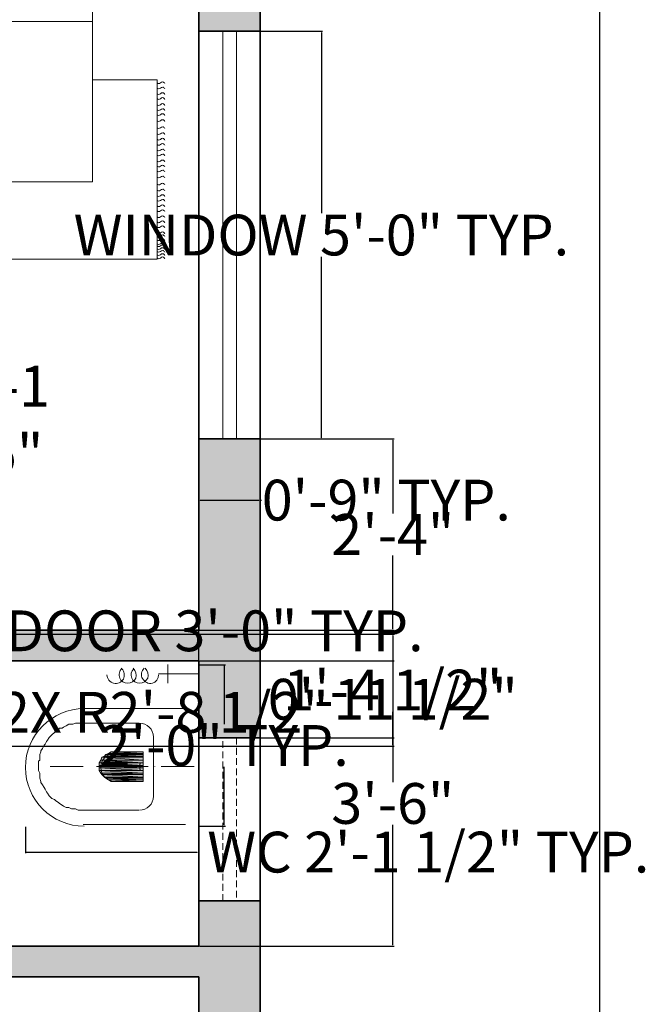
# Model space of a CAD drawing. Units: inches. Extents: x 335 to 688, y 1043 to 1486.
# Tile 6 of 7: x 596 to 688, y 1258 to 1403. Entities that reach past the tile are written whole.
import ezdxf

# ---------------------------------------------------------------- set-up
doc = ezdxf.new("R2010")
doc.units = ezdxf.units.IN
doc.header["$MEASUREMENT"] = 0
doc.linetypes.add('DASHEDX2', pattern=[1.5, 1, -0.5])
for name, color, linetype, lineweight in [('A-ANNO-DIMS', 2, 'Continuous', 18), ('A-ANNO-TTLB', 7, 'Continuous', 25), ('A-AREA-IDEN', 7, 'Continuous', 18), ('A-FLOR-FIXT', 8, 'Continuous', 18), ('A-FURN', 8, 'Continuous', 18), ('A-GLAZ', 4, 'Continuous', 18), ('A-GLAZ-VENT', 4, 'DASHEDX2', 18), ('A-WALL', 7, 'Continuous', 35), ('A-WALL-PATT', 252, 'Continuous', 13)]:
    doc.layers.add(name, color=color, linetype=linetype, lineweight=lineweight)
doc.styles.get("Standard").update_dxf_attribs({"font": 'arial.ttf'})
doc.dimstyles.get("Standard").update_dxf_attribs({"dimtxt": 6, "dimasz": 0.18, "dimexe": 0.18, "dimexo": 0.0625, "dimgap": 0.09, "dimtad": 0, "dimtih": 1, "dimtoh": 1, "dimdec": 1, "dimzin": 0, "dimdsep": 46, "dimlunit": 3, "dimtxsty": 'Standard', "dimcen": 0.09, "dimadec": 0, "dimazin": 0, "dimtfac": 1, "dimtdec": 1, "dimtofl": 0, "dimtmove": 0, "dimatfit": 3, "dimfxl": 1, "dimtolj": 1, "dimtzin": 0, "dimarcsym": 0})

# ---------------------------------------------------------------- blocks, each defined once
blk = doc.blocks.new('BED-DOUBLE-WITH-NIGHTSTANDS')
for p, q in [((56.59, 58.08), (56.59, 68.14)), ((0, 64.35), (26.37, 64.35)), ((0, 1.12), (0, 64.35)), ((26.37, 64.35), (26.37, 58.06)), ((61.62, 63.11), (51.56, 63.11)), ((34.96, 10.66), (34.96, 58.08)), ((52, 19.27), (52, 58.08)), ((52.82, 19.32), (52.82, 58.08)), ((52.82, 19.32), (46.47, 10.71)), ((52.82, 19.27), (46.47, 19.27)), ((46.47, 19.27), (46.47, 10.71)), ((26.37, 10.66), (26.37, 1.12)), ((56.69, 0.03), (56.69, 10.09)), ((61.72, 5.06), (51.66, 5.06)), ((26.37, 1.12), (0, 1.12))]:
    blk.add_line(p, q)
for points in [[(50.39, 68.71), (50.5, 58.08), (62.68, 58.08), (62.58, 68.71)], [(62.68, 10.66), (11.37, 10.66), (11.37, 58.08), (62.68, 58.08)], [(59.98, 38.83), (52.82, 38.83), (52.82, 52.73), (59.98, 52.73)], [(59.98, 19.27), (52.82, 19.27), (52.82, 33.16), (59.98, 33.16)], [(50.5, 10.66), (50.6, 0.03), (62.78, 0.03), (62.68, 10.66)]]:
    blk.add_lwpolyline(points, close=True)
for centre in [(56.59, 63.11), (56.69, 5.06)]:
    blk.add_circle(centre, 3.92)
for points, knots in [([(0.07, 65.48), (0.19, 65.39), (0.43, 65.19), (0.19, 64.85), (0.02, 64.57), (0.13, 64.42), (0.18, 64.35)], [0, 0, 0, 0, 0.400747, 0.791423, 1.067667, 1.29709, 1.29709, 1.29709, 1.29709]), ([(0.57, 65.48), (0.7, 65.39), (0.94, 65.19), (0.7, 64.85), (0.52, 64.57), (0.63, 64.42), (0.68, 64.35)], [0, 0, 0, 0, 0.400747, 0.791423, 1.067667, 1.29709, 1.29709, 1.29709, 1.29709]), ([(1.06, 65.48), (1.18, 65.39), (1.42, 65.19), (1.18, 64.85), (1.01, 64.57), (1.11, 64.42), (1.16, 64.35)], [0, 0, 0, 0, 0.400747, 0.791423, 1.067667, 1.29709, 1.29709, 1.29709, 1.29709]), ([(1.46, 65.48), (1.58, 65.39), (1.82, 65.19), (1.58, 64.85), (1.41, 64.57), (1.51, 64.42), (1.56, 64.35)], [0, 0, 0, 0, 0.400747, 0.791423, 1.067667, 1.29709, 1.29709, 1.29709, 1.29709]), ([(1.88, 65.48), (2, 65.39), (2.24, 65.19), (2, 64.85), (1.82, 64.57), (1.93, 64.42), (1.98, 64.35)], [0, 0, 0, 0, 0.400747, 0.791423, 1.067667, 1.29709, 1.29709, 1.29709, 1.29709]), ([(2.18, 65.48), (2.31, 65.39), (2.55, 65.19), (2.31, 64.85), (2.13, 64.57), (2.24, 64.42), (2.29, 64.35)], [0, 0, 0, 0, 0.400747, 0.791423, 1.067667, 1.29709, 1.29709, 1.29709, 1.29709]), ([(2.76, 65.48), (2.88, 65.39), (3.12, 65.19), (2.88, 64.85), (2.71, 64.57), (2.81, 64.42), (2.86, 64.35)], [0, 0, 0, 0, 0.400747, 0.791423, 1.067667, 1.29709, 1.29709, 1.29709, 1.29709]), ([(3.33, 65.48), (3.45, 65.39), (3.7, 65.19), (3.44, 64.85), (3.27, 64.57), (3.38, 64.42), (3.43, 64.35)], [0, 0, 0, 0, 0.407265, 0.802015, 1.07826, 1.307683, 1.307683, 1.307683, 1.307683]), ([(3.75, 65.48), (3.88, 65.39), (4.12, 65.19), (3.88, 64.85), (3.7, 64.57), (3.81, 64.42), (3.86, 64.35)], [0, 0, 0, 0, 0.400747, 0.791423, 1.067667, 1.29709, 1.29709, 1.29709, 1.29709]), ([(4.64, 65.48), (4.76, 65.39), (5, 65.19), (4.76, 64.85), (4.59, 64.57), (4.69, 64.42), (4.74, 64.35)], [0, 0, 0, 0, 0.400747, 0.791423, 1.067667, 1.29709, 1.29709, 1.29709, 1.29709]), ([(5.36, 65.48), (5.49, 65.39), (5.73, 65.19), (5.49, 64.85), (5.31, 64.57), (5.42, 64.42), (5.47, 64.35)], [0, 0, 0, 0, 0.400747, 0.791423, 1.067667, 1.29709, 1.29709, 1.29709, 1.29709]), ([(6.12, 65.48), (6.24, 65.39), (6.48, 65.19), (6.24, 64.85), (6.07, 64.57), (6.17, 64.42), (6.22, 64.35)], [0, 0, 0, 0, 0.400747, 0.791423, 1.067667, 1.29709, 1.29709, 1.29709, 1.29709]), ([(7, 65.48), (7.12, 65.39), (7.36, 65.19), (7.12, 64.85), (6.95, 64.57), (7.05, 64.42), (7.1, 64.35)], [0, 0, 0, 0, 0.400747, 0.791423, 1.067667, 1.29709, 1.29709, 1.29709, 1.29709]), ([(7.73, 65.48), (7.85, 65.39), (8.09, 65.19), (7.85, 64.85), (7.68, 64.57), (7.78, 64.42), (7.83, 64.35)], [0, 0, 0, 0, 0.400747, 0.791423, 1.067667, 1.29709, 1.29709, 1.29709, 1.29709]), ([(8.54, 65.48), (8.66, 65.39), (8.9, 65.19), (8.66, 64.85), (8.49, 64.57), (8.6, 64.42), (8.65, 64.35)], [0, 0, 0, 0, 0.400747, 0.791423, 1.067667, 1.29709, 1.29709, 1.29709, 1.29709]), ([(9.23, 65.48), (9.35, 65.39), (9.59, 65.19), (9.35, 64.85), (9.18, 64.57), (9.29, 64.42), (9.34, 64.35)], [0, 0, 0, 0, 0.400747, 0.791423, 1.067667, 1.29709, 1.29709, 1.29709, 1.29709]), ([(10.05, 65.48), (10.17, 65.39), (10.41, 65.19), (10.17, 64.85), (10, 64.57), (10.1, 64.42), (10.15, 64.35)], [0, 0, 0, 0, 0.400747, 0.791423, 1.067667, 1.29709, 1.29709, 1.29709, 1.29709]), ([(10.93, 65.48), (11.05, 65.39), (11.29, 65.19), (11.05, 64.85), (10.88, 64.57), (10.99, 64.42), (11.03, 64.35)], [0, 0, 0, 0, 0.400747, 0.791423, 1.067667, 1.29709, 1.29709, 1.29709, 1.29709]), ([(11.97, 65.48), (12.09, 65.39), (12.33, 65.19), (12.09, 64.85), (11.92, 64.57), (12.02, 64.42), (12.07, 64.35)], [0, 0, 0, 0, 0.400747, 0.791423, 1.067667, 1.29709, 1.29709, 1.29709, 1.29709]), ([(12.85, 65.48), (12.97, 65.39), (13.21, 65.19), (12.97, 64.85), (12.8, 64.57), (12.9, 64.42), (12.95, 64.35)], [0, 0, 0, 0, 0.400747, 0.791423, 1.067667, 1.29709, 1.29709, 1.29709, 1.29709]), ([(13.58, 65.48), (13.7, 65.39), (13.94, 65.19), (13.7, 64.85), (13.53, 64.57), (13.63, 64.42), (13.68, 64.35)], [0, 0, 0, 0, 0.400747, 0.791423, 1.067667, 1.29709, 1.29709, 1.29709, 1.29709]), ([(14.33, 65.48), (14.45, 65.39), (14.69, 65.19), (14.45, 64.85), (14.28, 64.57), (14.38, 64.42), (14.43, 64.35)], [0, 0, 0, 0, 0.400747, 0.791423, 1.067667, 1.29709, 1.29709, 1.29709, 1.29709]), ([(15.21, 65.48), (15.33, 65.39), (15.57, 65.19), (15.33, 64.85), (15.16, 64.57), (15.27, 64.42), (15.32, 64.35)], [0, 0, 0, 0, 0.400747, 0.791423, 1.067667, 1.29709, 1.29709, 1.29709, 1.29709]), ([(15.94, 65.48), (16.06, 65.39), (16.3, 65.19), (16.06, 64.85), (15.89, 64.57), (16, 64.42), (16.04, 64.35)], [0, 0, 0, 0, 0.400747, 0.791423, 1.067667, 1.29709, 1.29709, 1.29709, 1.29709]), ([(16.76, 65.48), (16.88, 65.39), (17.12, 65.19), (16.88, 64.85), (16.7, 64.57), (16.81, 64.42), (16.86, 64.35)], [0, 0, 0, 0, 0.400747, 0.791423, 1.067667, 1.29709, 1.29709, 1.29709, 1.29709]), ([(17.53, 65.48), (17.65, 65.39), (17.89, 65.19), (17.65, 64.85), (17.48, 64.57), (17.59, 64.42), (17.64, 64.35)], [0, 0, 0, 0, 0.400747, 0.791423, 1.067667, 1.29709, 1.29709, 1.29709, 1.29709]), ([(18.35, 65.48), (18.47, 65.39), (18.71, 65.19), (18.47, 64.85), (18.3, 64.57), (18.4, 64.42), (18.45, 64.35)], [0, 0, 0, 0, 0.400747, 0.791423, 1.067667, 1.29709, 1.29709, 1.29709, 1.29709]), ([(19.23, 65.48), (19.35, 65.39), (19.59, 65.19), (19.35, 64.85), (19.18, 64.57), (19.29, 64.42), (19.33, 64.35)], [0, 0, 0, 0, 0.400747, 0.791423, 1.067667, 1.29709, 1.29709, 1.29709, 1.29709]), ([(20.27, 65.48), (20.39, 65.39), (20.63, 65.19), (20.39, 64.85), (20.22, 64.57), (20.32, 64.42), (20.37, 64.35)], [0, 0, 0, 0, 0.400747, 0.791423, 1.067667, 1.29709, 1.29709, 1.29709, 1.29709]), ([(21.15, 65.48), (21.27, 65.39), (21.51, 65.19), (21.27, 64.85), (21.1, 64.57), (21.21, 64.42), (21.25, 64.35)], [0, 0, 0, 0, 0.400747, 0.791423, 1.067667, 1.29709, 1.29709, 1.29709, 1.29709]), ([(21.88, 65.48), (22, 65.39), (22.24, 65.19), (22, 64.85), (21.83, 64.57), (21.93, 64.42), (21.98, 64.35)], [0, 0, 0, 0, 0.400747, 0.791423, 1.067667, 1.29709, 1.29709, 1.29709, 1.29709]), ([(22.63, 65.48), (22.75, 65.39), (22.99, 65.19), (22.75, 64.85), (22.58, 64.57), (22.69, 64.42), (22.73, 64.35)], [0, 0, 0, 0, 0.400747, 0.791423, 1.067667, 1.29709, 1.29709, 1.29709, 1.29709]), ([(23.51, 65.48), (23.63, 65.39), (23.87, 65.19), (23.63, 64.85), (23.46, 64.57), (23.57, 64.42), (23.62, 64.35)], [0, 0, 0, 0, 0.400747, 0.791423, 1.067667, 1.29709, 1.29709, 1.29709, 1.29709]), ([(24.24, 65.48), (24.36, 65.39), (24.6, 65.19), (24.36, 64.85), (24.19, 64.57), (24.3, 64.42), (24.34, 64.35)], [0, 0, 0, 0, 0.400747, 0.791423, 1.067667, 1.29709, 1.29709, 1.29709, 1.29709]), ([(25.06, 65.48), (25.18, 65.39), (25.42, 65.19), (25.18, 64.85), (25.01, 64.57), (25.11, 64.42), (25.16, 64.35)], [0, 0, 0, 0, 0.400747, 0.791423, 1.067667, 1.29709, 1.29709, 1.29709, 1.29709]), ([(25.84, 65.48), (25.96, 65.39), (26.2, 65.19), (25.96, 64.85), (25.78, 64.57), (25.89, 64.42), (25.94, 64.35)], [0, 0, 0, 0, 0.400747, 0.791423, 1.067667, 1.29709, 1.29709, 1.29709, 1.29709]), ([(0.07, 0), (0.19, 0.1), (0.43, 0.29), (0.19, 0.63), (0.02, 0.91), (0.13, 1.06), (0.18, 1.13)], [0, 0, 0, 0, 0.400747, 0.791423, 1.067667, 1.29709, 1.29709, 1.29709, 1.29709]), ([(0.55, 0), (0.67, 0.1), (0.91, 0.29), (0.67, 0.63), (0.49, 0.91), (0.6, 1.06), (0.65, 1.13)], [0, 0, 0, 0, 0.400747, 0.791423, 1.067667, 1.29709, 1.29709, 1.29709, 1.29709]), ([(1.03, 0), (1.15, 0.1), (1.39, 0.29), (1.15, 0.63), (0.98, 0.91), (1.09, 1.06), (1.13, 1.13)], [0, 0, 0, 0, 0.400747, 0.791423, 1.067667, 1.29709, 1.29709, 1.29709, 1.29709]), ([(1.43, 0), (1.55, 0.1), (1.79, 0.29), (1.55, 0.63), (1.38, 0.91), (1.48, 1.06), (1.53, 1.13)], [0, 0, 0, 0, 0.400747, 0.791423, 1.067667, 1.29709, 1.29709, 1.29709, 1.29709]), ([(1.85, 0), (1.97, 0.1), (2.21, 0.29), (1.97, 0.63), (1.8, 0.91), (1.9, 1.05), (1.94, 1.12)], [0, 0, 0, 0, 0.400747, 0.791423, 1.067667, 1.283686, 1.283686, 1.283686, 1.283686]), ([(2.16, 0), (2.28, 0.1), (2.52, 0.29), (2.28, 0.63), (2.11, 0.91), (2.21, 1.05), (2.25, 1.12)], [0, 0, 0, 0, 0.400747, 0.791423, 1.067667, 1.283686, 1.283686, 1.283686, 1.283686]), ([(2.73, 0), (2.85, 0.1), (3.09, 0.29), (2.85, 0.63), (2.68, 0.91), (2.78, 1.05), (2.82, 1.12)], [0, 0, 0, 0, 0.400747, 0.791423, 1.067667, 1.283686, 1.283686, 1.283686, 1.283686]), ([(3.33, 0), (3.45, 0.1), (3.69, 0.29), (3.45, 0.63), (3.28, 0.91), (3.38, 1.05), (3.42, 1.12)], [0, 0, 0, 0, 0.402903, 0.794912, 1.071156, 1.287177, 1.287177, 1.287177, 1.287177]), ([(3.75, 0), (3.88, 0.1), (4.12, 0.29), (3.88, 0.63), (3.7, 0.91), (3.81, 1.05), (3.85, 1.12)], [0, 0, 0, 0, 0.400747, 0.791423, 1.067667, 1.283686, 1.283686, 1.283686, 1.283686]), ([(4.64, 0), (4.76, 0.1), (5, 0.29), (4.76, 0.63), (4.59, 0.91), (4.69, 1.05), (4.73, 1.12)], [0, 0, 0, 0, 0.400747, 0.791423, 1.067667, 1.283686, 1.283686, 1.283686, 1.283686]), ([(5.36, 0), (5.49, 0.1), (5.73, 0.29), (5.49, 0.63), (5.31, 0.91), (5.42, 1.06), (5.47, 1.13)], [0, 0, 0, 0, 0.400747, 0.791423, 1.067667, 1.29709, 1.29709, 1.29709, 1.29709]), ([(6.12, 0), (6.24, 0.1), (6.48, 0.29), (6.24, 0.63), (6.07, 0.91), (6.17, 1.06), (6.22, 1.13)], [0, 0, 0, 0, 0.400747, 0.791423, 1.067667, 1.29709, 1.29709, 1.29709, 1.29709]), ([(7, 0), (7.12, 0.1), (7.36, 0.29), (7.12, 0.63), (6.95, 0.91), (7.05, 1.06), (7.1, 1.13)], [0, 0, 0, 0, 0.400747, 0.791423, 1.067667, 1.29709, 1.29709, 1.29709, 1.29709]), ([(7.73, 0), (7.85, 0.1), (8.09, 0.29), (7.85, 0.63), (7.68, 0.91), (7.78, 1.06), (7.83, 1.13)], [0, 0, 0, 0, 0.400747, 0.791423, 1.067667, 1.29709, 1.29709, 1.29709, 1.29709]), ([(8.54, 0), (8.66, 0.1), (8.9, 0.29), (8.66, 0.63), (8.49, 0.91), (8.6, 1.06), (8.65, 1.13)], [0, 0, 0, 0, 0.400747, 0.791423, 1.067667, 1.29709, 1.29709, 1.29709, 1.29709]), ([(9.23, 0), (9.35, 0.1), (9.59, 0.29), (9.35, 0.63), (9.18, 0.91), (9.29, 1.06), (9.34, 1.13)], [0, 0, 0, 0, 0.400747, 0.791423, 1.067667, 1.29709, 1.29709, 1.29709, 1.29709]), ([(10.05, 0), (10.17, 0.1), (10.41, 0.29), (10.17, 0.63), (10, 0.91), (10.1, 1.06), (10.15, 1.13)], [0, 0, 0, 0, 0.400747, 0.791423, 1.067667, 1.29709, 1.29709, 1.29709, 1.29709]), ([(10.93, 0), (11.05, 0.1), (11.29, 0.29), (11.05, 0.63), (10.88, 0.91), (10.99, 1.06), (11.03, 1.13)], [0, 0, 0, 0, 0.400747, 0.791423, 1.067667, 1.29709, 1.29709, 1.29709, 1.29709]), ([(11.97, 0), (12.09, 0.1), (12.33, 0.29), (12.09, 0.63), (11.92, 0.91), (12.02, 1.06), (12.07, 1.13)], [0, 0, 0, 0, 0.400747, 0.791423, 1.067667, 1.29709, 1.29709, 1.29709, 1.29709]), ([(12.85, 0), (12.97, 0.1), (13.21, 0.29), (12.97, 0.63), (12.8, 0.91), (12.9, 1.06), (12.95, 1.13)], [0, 0, 0, 0, 0.400747, 0.791423, 1.067667, 1.29709, 1.29709, 1.29709, 1.29709]), ([(13.58, 0), (13.7, 0.1), (13.94, 0.29), (13.7, 0.63), (13.53, 0.91), (13.63, 1.06), (13.68, 1.13)], [0, 0, 0, 0, 0.400747, 0.791423, 1.067667, 1.29709, 1.29709, 1.29709, 1.29709]), ([(14.33, 0), (14.45, 0.1), (14.69, 0.29), (14.45, 0.63), (14.28, 0.91), (14.38, 1.06), (14.43, 1.13)], [0, 0, 0, 0, 0.400747, 0.791423, 1.067667, 1.29709, 1.29709, 1.29709, 1.29709]), ([(15.21, 0), (15.33, 0.1), (15.57, 0.29), (15.33, 0.63), (15.16, 0.91), (15.27, 1.06), (15.32, 1.13)], [0, 0, 0, 0, 0.400747, 0.791423, 1.067667, 1.29709, 1.29709, 1.29709, 1.29709]), ([(15.94, 0), (16.06, 0.1), (16.3, 0.29), (16.06, 0.63), (15.89, 0.91), (16, 1.06), (16.04, 1.13)], [0, 0, 0, 0, 0.400747, 0.791423, 1.067667, 1.29709, 1.29709, 1.29709, 1.29709]), ([(16.76, 0), (16.88, 0.1), (17.12, 0.29), (16.88, 0.63), (16.7, 0.91), (16.81, 1.06), (16.86, 1.13)], [0, 0, 0, 0, 0.400747, 0.791423, 1.067667, 1.29709, 1.29709, 1.29709, 1.29709]), ([(17.53, 0), (17.65, 0.1), (17.89, 0.29), (17.65, 0.63), (17.48, 0.91), (17.59, 1.06), (17.64, 1.13)], [0, 0, 0, 0, 0.400747, 0.791423, 1.067667, 1.29709, 1.29709, 1.29709, 1.29709]), ([(18.35, 0), (18.47, 0.1), (18.71, 0.29), (18.47, 0.63), (18.3, 0.91), (18.4, 1.06), (18.45, 1.13)], [0, 0, 0, 0, 0.400747, 0.791423, 1.067667, 1.29709, 1.29709, 1.29709, 1.29709]), ([(19.23, 0), (19.35, 0.1), (19.59, 0.29), (19.35, 0.63), (19.18, 0.91), (19.29, 1.06), (19.33, 1.13)], [0, 0, 0, 0, 0.400747, 0.791423, 1.067667, 1.29709, 1.29709, 1.29709, 1.29709]), ([(20.27, 0), (20.39, 0.1), (20.63, 0.29), (20.39, 0.63), (20.22, 0.91), (20.32, 1.06), (20.37, 1.13)], [0, 0, 0, 0, 0.400747, 0.791423, 1.067667, 1.29709, 1.29709, 1.29709, 1.29709]), ([(21.15, 0), (21.27, 0.1), (21.51, 0.29), (21.27, 0.63), (21.1, 0.91), (21.21, 1.06), (21.25, 1.13)], [0, 0, 0, 0, 0.400747, 0.791423, 1.067667, 1.29709, 1.29709, 1.29709, 1.29709]), ([(21.88, 0), (22, 0.1), (22.24, 0.29), (22, 0.63), (21.83, 0.91), (21.93, 1.06), (21.98, 1.13)], [0, 0, 0, 0, 0.400747, 0.791423, 1.067667, 1.29709, 1.29709, 1.29709, 1.29709]), ([(22.63, 0), (22.75, 0.1), (22.99, 0.29), (22.75, 0.63), (22.58, 0.91), (22.69, 1.06), (22.73, 1.13)], [0, 0, 0, 0, 0.400747, 0.791423, 1.067667, 1.29709, 1.29709, 1.29709, 1.29709]), ([(23.51, 0), (23.63, 0.1), (23.87, 0.29), (23.63, 0.63), (23.46, 0.91), (23.57, 1.06), (23.62, 1.13)], [0, 0, 0, 0, 0.400747, 0.791423, 1.067667, 1.29709, 1.29709, 1.29709, 1.29709]), ([(24.24, 0), (24.36, 0.1), (24.6, 0.29), (24.36, 0.63), (24.19, 0.91), (24.3, 1.06), (24.34, 1.13)], [0, 0, 0, 0, 0.400747, 0.791423, 1.067667, 1.29709, 1.29709, 1.29709, 1.29709]), ([(25.06, 0), (25.18, 0.1), (25.42, 0.29), (25.18, 0.63), (25.01, 0.91), (25.11, 1.06), (25.16, 1.13)], [0, 0, 0, 0, 0.400747, 0.791423, 1.067667, 1.29709, 1.29709, 1.29709, 1.29709]), ([(25.84, 0), (25.96, 0.1), (26.2, 0.29), (25.96, 0.63), (25.78, 0.91), (25.89, 1.06), (25.94, 1.13)], [0, 0, 0, 0, 0.400747, 0.791423, 1.067667, 1.29709, 1.29709, 1.29709, 1.29709])]:
    blk.add_open_spline(points, degree=3, knots=knots)
blk = doc.blocks.new('WC')
h = blk.add_hatch(color=256)
h.paths.add_polyline_path([(17.3, 10.16), (11.23, 10.16), (17.3, 9.71)])
h.paths.add_polyline_path([(11.23, 10.16), (17.3, 9.71), (11.08, 9.71)])
h = blk.add_hatch(color=256)
h.paths.add_polyline_path([(17.3, 10.32), (11.61, 10.32), (17.3, 10.16)])
h.paths.add_polyline_path([(11.61, 10.32), (17.3, 10.16), (11.23, 10.16)])
h = blk.add_hatch(color=256)
h.paths.add_polyline_path([(17.3, 10.54), (11.83, 10.54), (17.3, 10.32)])
h.paths.add_polyline_path([(11.83, 10.54), (17.3, 10.32), (11.61, 10.32)])
h = blk.add_hatch(color=256)
h.paths.add_polyline_path([(17.3, 10.7), (12.21, 10.7), (17.3, 10.54)])
h.paths.add_polyline_path([(12.21, 10.7), (17.3, 10.54), (11.83, 10.54)])
h = blk.add_hatch(color=256)
h.paths.add_polyline_path([(17.3, 10.92), (12.59, 10.92), (17.3, 10.7)])
h.paths.add_polyline_path([(12.59, 10.92), (17.3, 10.7), (12.21, 10.7)])
h = blk.add_hatch(color=256)
h.paths.add_polyline_path([(17.3, 9.71), (11.08, 9.71), (17.3, 9.33)])
h.paths.add_polyline_path([(11.08, 9.71), (17.3, 9.33), (10.85, 9.33)])
h = blk.add_hatch(color=256)
h.paths.add_polyline_path([(17.3, 9.33), (10.85, 9.33), (17.3, 8.95)])
h.paths.add_polyline_path([(10.85, 9.33), (17.3, 8.95), (10.85, 8.95)])
h = blk.add_hatch(color=256)
h.paths.add_polyline_path([(17.3, 8.95), (10.85, 8.95), (17.3, 8.57)])
h.paths.add_polyline_path([(10.85, 8.95), (17.3, 8.57), (10.85, 8.57)])
h = blk.add_hatch(color=256)
h.paths.add_polyline_path([(17.3, 8.57), (10.85, 8.57), (17.3, 8.19)])
h.paths.add_polyline_path([(10.85, 8.57), (17.3, 8.19), (10.85, 8.19)])
h = blk.add_hatch(color=256)
h.paths.add_polyline_path([(17.3, 8.19), (10.85, 8.19), (17.3, 7.81)])
h.paths.add_polyline_path([(10.85, 8.19), (17.3, 7.81), (11.08, 7.81)])
h = blk.add_hatch(color=256)
h.paths.add_polyline_path([(17.3, 7.81), (11.08, 7.81), (17.3, 7.59)])
h.paths.add_polyline_path([(11.08, 7.81), (17.3, 7.59), (11.23, 7.59)])
h = blk.add_hatch(color=256)
h.paths.add_polyline_path([(17.3, 7.59), (11.23, 7.59), (17.3, 7.21)])
h.paths.add_polyline_path([(11.23, 7.59), (17.3, 7.21), (11.61, 7.21)])
h = blk.add_hatch(color=256)
h.paths.add_polyline_path([(17.3, 7.21), (11.61, 7.21), (17.3, 7.05)])
h.paths.add_polyline_path([(11.61, 7.21), (17.3, 7.05), (11.83, 7.05)])
h = blk.add_hatch(color=256)
h.paths.add_polyline_path([(17.3, 7.05), (11.83, 7.05), (17.3, 6.83)])
h.paths.add_polyline_path([(11.83, 7.05), (17.3, 6.83), (12.21, 6.83)])
h = blk.add_hatch(color=256)
h.paths.add_polyline_path([(17.3, 6.83), (12.21, 6.83), (17.3, 6.6)])
h.paths.add_polyline_path([(12.21, 6.83), (17.3, 6.6), (12.59, 6.6)])
h.paths.add_polyline_path([(17.3, 6.6), (12.59, 6.6), (12.97, 6.6)])
for points in [[(20.94, 21.04), (20.94, 23.77), (20.94, 23.77)], [(25.41, 22.4), (19.57, 22.4), (19.57, 22.4)], [(23.52, 17.3), (8.5, 17.3), (8.5, 17.3)], [(9.48, 2.35), (8.72, 2.35), (8.12, 2.35), (7.74, 2.35), (7.36, 2.58), (6.98, 2.58), (6.75, 2.58), (6.37, 2.73), (5.99, 2.73), (5.61, 2.96), (5.39, 3.11), (5.01, 3.34), (4.85, 3.49), (4.48, 3.72), (4.25, 3.94), (3.87, 4.1), (3.64, 4.32), (3.49, 4.48), (3.26, 4.85), (3.11, 5.08), (2.88, 5.46), (2.73, 5.69), (2.5, 6.07), (2.28, 6.45), (2.28, 6.6), (2.12, 7.05), (2.12, 7.43), (2.12, 7.81), (1.9, 8.19), (1.9, 8.8), (1.9, 9.56), (2.12, 9.71), (2.12, 10.16), (2.12, 10.54), (2.28, 10.92), (2.28, 11.08), (2.5, 11.45), (2.73, 11.91), (2.88, 12.06), (3.11, 12.44), (3.26, 12.67), (3.49, 13.05), (3.64, 13.2), (3.87, 13.43), (4.25, 13.81), (4.48, 14.03), (4.85, 14.19), (5.01, 14.41), (5.39, 14.41), (5.61, 14.56), (5.99, 14.79), (6.37, 15.02), (6.75, 15.02), (6.98, 15.02), (7.36, 15.17), (7.74, 15.17), (8.12, 15.17), (8.72, 15.17), (9.48, 15.17)], [(16.69, 15.17), (9.48, 15.17), (9.48, 15.17)], [(18.81, 4.48), (18.81, 13.2), (18.81, 13.2)], [(17.3, 10.92), (12.97, 10.92), (12.97, 10.92)], [(17.3, 6.6), (17.3, 10.92), (17.3, 10.92)], [(8.5, 8.8), (3.64, 8.8), (3.64, 8.8)], [(18.05, 8.8), (10.47, 8.8), (10.47, 8.8)], [(16.84, 9.18), (16.92, 9.18), (16.92, 9.18)], [(16.84, 8.8), (16.84, 8.95), (16.84, 9.18)], [(16.84, 8.8), (16.92, 8.72), (16.92, 8.72)], [(16.84, 8.34), (16.84, 8.57), (16.84, 8.8)], [(19.04, 8.8), (19.04, 8.72), (19.04, 8.72)], [(24.81, 8.8), (19.95, 8.8), (19.95, 8.8)], [(16.84, 8.34), (16.92, 8.34), (16.92, 8.34)], [(17.3, 6.6), (12.97, 6.6), (12.97, 6.6)], [(16.69, 2.35), (9.48, 2.35), (9.48, 2.35)], [(23.52, 0.23), (8.5, 0.23), (8.5, 0.23)]]:
    blk.add_lwpolyline(points)
for points in [[(11.23, 10.16), (17.3, 9.71), (11.08, 9.71)], [(11.61, 10.32), (17.3, 10.16), (11.23, 10.16)], [(17.3, 10.16), (11.23, 10.16), (17.3, 9.71)], [(11.83, 10.54), (17.3, 10.32), (11.61, 10.32)], [(17.3, 10.32), (11.61, 10.32), (17.3, 10.16)], [(12.21, 10.7), (17.3, 10.54), (11.83, 10.54)], [(17.3, 10.54), (11.83, 10.54), (17.3, 10.32)], [(12.59, 10.92), (17.3, 10.7), (12.21, 10.7)], [(17.3, 10.7), (12.21, 10.7), (17.3, 10.54)], [(12.97, 10.92), (17.3, 10.92), (12.59, 10.92)], [(17.3, 10.92), (12.59, 10.92), (17.3, 10.7)], [(17.3, 10.92), (12.97, 10.92)], [(11.08, 9.71), (17.3, 9.33), (10.85, 9.33)], [(17.3, 9.33), (10.85, 9.33), (17.3, 8.95)], [(10.85, 9.33), (17.3, 8.95), (10.85, 8.95)], [(17.3, 8.95), (10.85, 8.95), (17.3, 8.57)], [(10.85, 8.95), (17.3, 8.57), (10.85, 8.57)], [(17.3, 9.71), (11.08, 9.71), (17.3, 9.33)], [(17.3, 8.57), (10.85, 8.57), (17.3, 8.19)], [(10.85, 8.57), (17.3, 8.19), (10.85, 8.19)], [(17.3, 8.19), (10.85, 8.19), (17.3, 7.81)], [(10.85, 8.19), (17.3, 7.81), (11.08, 7.81)], [(17.3, 7.81), (11.08, 7.81), (17.3, 7.59)], [(11.08, 7.81), (17.3, 7.59), (11.23, 7.59)], [(17.3, 7.59), (11.23, 7.59), (17.3, 7.21)], [(11.23, 7.59), (17.3, 7.21), (11.61, 7.21)], [(17.3, 7.21), (11.61, 7.21), (17.3, 7.05)], [(11.61, 7.21), (17.3, 7.05), (11.83, 7.05)], [(17.3, 7.05), (11.83, 7.05), (17.3, 6.83)], [(11.83, 7.05), (17.3, 6.83), (12.21, 6.83)], [(17.3, 6.83), (12.21, 6.83), (17.3, 6.6)], [(12.21, 6.83), (17.3, 6.6), (12.59, 6.6)], [(17.3, 6.6), (12.59, 6.6), (12.97, 6.6)], [(12.59, 6.6), (17.3, 6.6), (17.3, 6.6)]]:
    blk.add_lwpolyline(points, close=True)
for points, knots in [([(14.19, 23.23), (13.81, 22.86), (13.65, 22.32), (13.88, 21.79), (13.88, 21.79), (14.03, 21.34), (14.49, 21.04), (15.02, 21.04), (15.02, 21.04), (15.55, 21.04), (16.01, 21.34), (16.23, 21.79), (16.23, 21.79), (16.39, 22.32), (16.23, 22.86), (15.85, 23.23)], [0, 0, 0, 0, 0.0625, 0.0625, 0.0625, 0.062501, 0.125, 0.125, 0.125, 0.125001, 0.1875, 0.1875, 0.1875, 0.187501, 1, 1, 1, 1]), ([(15.93, 23.16), (15.55, 22.86), (15.4, 22.25), (15.63, 21.79), (15.63, 21.79), (15.78, 21.34), (16.31, 21.04), (16.76, 21.04), (16.76, 21.04), (17.3, 21.04), (17.75, 21.34), (17.98, 21.79), (17.98, 21.79), (18.13, 22.32), (17.98, 22.86), (17.6, 23.23)], [0, 0, 0, 0, 0.0625, 0.0625, 0.0625, 0.062501, 0.125, 0.125, 0.125, 0.125001, 0.1875, 0.1875, 0.1875, 0.187501, 1, 1, 1, 1]), ([(17.45, 23.23), (17.07, 22.86), (16.92, 22.17), (17.22, 21.72), (17.22, 21.72), (17.52, 21.19), (18.05, 20.88), (18.66, 21.04), (18.66, 21.04), (19.19, 21.19), (19.57, 21.72), (19.57, 22.25)], [0, 0, 0, 0, 0.083333, 0.083333, 0.083333, 0.083334, 0.166667, 0.166667, 0.166667, 0.166668, 1, 1, 1, 1]), ([(11.99, 22.25), (11.99, 21.72), (12.44, 21.19), (12.97, 21.04), (12.97, 21.04), (13.5, 20.88), (14.11, 21.19), (14.41, 21.64), (14.41, 21.64), (14.64, 22.17), (14.56, 22.78), (14.19, 23.16)], [0, 0, 0, 0, 0.083333, 0.083333, 0.083333, 0.083334, 0.166667, 0.166667, 0.166667, 0.166668, 1, 1, 1, 1]), ([(8.65, 17.3), (3.87, 17.3), (0, 13.43), (0, 8.65), (0, 8.65), (0, 3.87), (3.87, 0), (8.65, 0)], [0, 0, 0, 0, 0.125, 0.125, 0.125, 0.125001, 1, 1, 1, 1]), ([(13.12, 10.7), (11.99, 10.7), (11.08, 9.79), (11.08, 8.65), (11.08, 8.65), (11.08, 7.51), (11.99, 6.6), (13.12, 6.6)], [0, 0, 0, 0, 0.125, 0.125, 0.125, 0.125001, 1, 1, 1, 1])]:
    blk.add_open_spline(points, degree=3, knots=knots)
for points in [[(18.81, 13.12), (18.81, 14.26), (17.9, 15.17), (16.76, 15.17)], [(16.76, 2.35), (17.9, 2.35), (18.81, 3.26), (18.81, 4.4)]]:
    blk.add_open_spline(points, degree=3)
blk = doc.blocks.new('WIN-60IN')
for p, q in [((0, 0), (0, 60)), ((3.5, 0), (3.5, 60)), ((5.5, 60), (5.5, 0)), ((9, 60), (9, 0))]:
    blk.add_line(p, q)
blk = doc.blocks.new('VENT-24IN')
for p, q in [((0, 0), (0, 24)), ((3.5, 0), (3.5, 24)), ((5.5, 24), (5.5, 0)), ((9, 24), (9, 0))]:
    blk.add_line(p, q)
blk = doc.blocks.new('*D17')
at = {"layer": 'A-ANNO-DIMS', "color": 0, "lineweight": -2, "transparency": 16777216}
for p, q in [((596.6, 1284.55), (596.6, 1280.63)), ((622.02, 1284.55), (622.02, 1280.63)), ((596.78, 1280.81), (621.84, 1280.81)), ((622.02, 1280.81), (622.2, 1280.81))]:
    blk.add_line(p, q, dxfattribs=at)
at = {"layer": 'A-ANNO-DIMS', "color": 0, "transparency": 16777216}
for points in [[(596.78, 1280.84), (596.78, 1280.78), (596.6, 1280.81)], [(621.84, 1280.84), (621.84, 1280.78), (622.02, 1280.81)]]:
    blk.add_solid(points, dxfattribs=at)
at = {"layer": 'Defpoints', "color": 0, "transparency": 16777216}
for p in [(596.6, 1284.62), (622.02, 1284.62), (622.02, 1280.81)]:
    blk.add_point(p, dxfattribs=at)
at = {"layer": 'A-ANNO-DIMS', "color": 0, "transparency": 16777216, "insert": (655.83, 1280.81), "char_height": 6, "attachment_point": 5}
blk.add_mtext('\\A1;WC 2\'-1 1/2" TYP.', dxfattribs=at)
blk = doc.blocks.new('*D18')
at = {"layer": 'A-ANNO-DIMS', "color": 0, "lineweight": -2, "transparency": 16777216}
for p, q in [((622.08, 1308.38), (626.01, 1308.38)), ((625.83, 1308.2), (625.83, 1299.65)), ((625.83, 1284.8), (625.83, 1293.35)), ((622.08, 1284.62), (626.01, 1284.62))]:
    blk.add_line(p, q, dxfattribs=at)
at = {"layer": 'A-ANNO-DIMS', "color": 0, "transparency": 16777216}
for points in [[(625.8, 1308.2), (625.86, 1308.2), (625.83, 1308.38)], [(625.8, 1284.8), (625.86, 1284.8), (625.83, 1284.62)]]:
    blk.add_solid(points, dxfattribs=at)
at = {"layer": 'Defpoints', "color": 0, "transparency": 16777216}
for p in [(622.02, 1308.38), (625.83, 1308.38), (622.02, 1284.62)]:
    blk.add_point(p, dxfattribs=at)
at = {"layer": 'A-ANNO-DIMS', "color": 0, "transparency": 16777216, "insert": (625.83, 1296.5), "char_height": 6, "attachment_point": 5}
blk.add_mtext('\\A1;2\'-0" TYP.', dxfattribs=at)
blk = doc.blocks.new('*D25')
at = {"layer": 'A-ANNO-DIMS', "color": 0, "lineweight": -2, "transparency": 16777216}
for p, q in [((631.17, 1401.6), (640.29, 1401.6)), ((640.11, 1401.42), (640.11, 1374.8)), ((640.11, 1341.78), (640.11, 1368.41)), ((631.17, 1341.6), (640.29, 1341.6))]:
    blk.add_line(p, q, dxfattribs=at)
at = {"layer": 'A-ANNO-DIMS', "color": 0, "transparency": 16777216}
for points in [[(640.08, 1401.42), (640.14, 1401.42), (640.11, 1401.6)], [(640.08, 1341.78), (640.14, 1341.78), (640.11, 1341.6)]]:
    blk.add_solid(points, dxfattribs=at)
at = {"layer": 'Defpoints', "color": 0, "transparency": 16777216}
for p in [(631.11, 1401.6), (640.11, 1401.6), (631.11, 1341.6)]:
    blk.add_point(p, dxfattribs=at)
at = {"layer": 'A-ANNO-DIMS', "color": 0, "transparency": 16777216, "insert": (640.11, 1371.6), "char_height": 6, "attachment_point": 5}
blk.add_mtext('\\A1;WINDOW 5\'-0" TYP.', dxfattribs=at)
blk = doc.blocks.new('*D26')
at = {"layer": 'A-ANNO-DIMS', "color": 0, "lineweight": -2, "transparency": 16777216}
for p, q in [((622.11, 1341.54), (622.11, 1332.42)), ((631.11, 1341.54), (631.11, 1332.42)), ((622.29, 1332.6), (630.93, 1332.6)), ((631.11, 1332.6), (631.29, 1332.6))]:
    blk.add_line(p, q, dxfattribs=at)
at = {"layer": 'A-ANNO-DIMS', "color": 0, "transparency": 16777216}
for points in [[(622.29, 1332.63), (622.29, 1332.57), (622.11, 1332.6)], [(630.93, 1332.63), (630.93, 1332.57), (631.11, 1332.6)]]:
    blk.add_solid(points, dxfattribs=at)
at = {"layer": 'Defpoints', "color": 0, "transparency": 16777216}
for p in [(622.11, 1341.6), (631.11, 1341.6), (631.11, 1332.6)]:
    blk.add_point(p, dxfattribs=at)
at = {"layer": 'A-ANNO-DIMS', "color": 0, "transparency": 16777216, "insert": (649.66, 1332.6), "char_height": 6, "attachment_point": 5}
blk.add_mtext('\\A1;0\'-9" TYP.', dxfattribs=at)
blk = doc.blocks.new('*D31')
at = {"layer": 'A-ANNO-DIMS', "color": 0, "lineweight": -2, "transparency": 16777216}
for p, q in [((512.61, 1308.03), (512.61, 1313.55)), ((512.79, 1313.37), (548.43, 1313.37)), ((548.61, 1308.03), (548.61, 1313.55)), ((548.61, 1313.37), (548.79, 1313.37))]:
    blk.add_line(p, q, dxfattribs=at)
at = {"layer": 'A-ANNO-DIMS', "color": 0, "transparency": 16777216}
for points in [[(512.79, 1313.4), (512.79, 1313.34), (512.61, 1313.37)], [(548.43, 1313.4), (548.43, 1313.34), (548.61, 1313.37)]]:
    blk.add_solid(points, dxfattribs=at)
at = {"layer": 'Defpoints', "color": 0, "transparency": 16777216}
for p in [(548.61, 1313.37), (512.61, 1307.97), (548.61, 1307.97)]:
    blk.add_point(p, dxfattribs=at)
at = {"layer": 'A-ANNO-DIMS', "color": 0, "transparency": 16777216, "insert": (603.59, 1313.37), "char_height": 6, "attachment_point": 5}
blk.add_mtext('\\A1;BEDROOM DOOR 3\'-0" TYP.', dxfattribs=at)
blk = doc.blocks.new('*D41')
at = {"layer": 'A-ANNO-DIMS', "color": 0, "lineweight": -2, "transparency": 16777216}
for p, q in [((430.31, 1312.88), (650.79, 1312.88)), ((650.61, 1312.7), (650.61, 1307.84)), ((650.61, 1296.6), (650.61, 1301.46)), ((430.31, 1296.42), (650.79, 1296.42))]:
    blk.add_line(p, q, dxfattribs=at)
at = {"layer": 'A-ANNO-DIMS', "color": 0, "transparency": 16777216}
for points in [[(650.58, 1312.7), (650.64, 1312.7), (650.61, 1312.88)], [(650.58, 1296.6), (650.64, 1296.6), (650.61, 1296.42)]]:
    blk.add_solid(points, dxfattribs=at)
at = {"layer": 'Defpoints', "color": 0, "transparency": 16777216}
for p in [(430.25, 1312.88), (650.61, 1312.88), (430.25, 1296.42)]:
    blk.add_point(p, dxfattribs=at)
at = {"layer": 'A-ANNO-DIMS', "color": 0, "transparency": 16777216, "insert": (650.61, 1304.65), "char_height": 6, "attachment_point": 5}
blk.add_mtext('\\A1;1\'-4 1/2"', dxfattribs=at)
blk = doc.blocks.new('*D42')
at = {"layer": 'A-ANNO-DIMS', "color": 0, "lineweight": -2, "transparency": 16777216}
for p, q in [((557.61, 1309.03), (557.61, 1460.65)), ((557.79, 1460.47), (574.8, 1460.47)), ((621.93, 1460.47), (604.91, 1460.47)), ((622.11, 1309.03), (622.11, 1460.65))]:
    blk.add_line(p, q, dxfattribs=at)
at = {"layer": 'A-ANNO-DIMS', "color": 0, "transparency": 16777216}
for points in [[(557.79, 1460.5), (557.79, 1460.44), (557.61, 1460.47)], [(621.93, 1460.5), (621.93, 1460.44), (622.11, 1460.47)]]:
    blk.add_solid(points, dxfattribs=at)
at = {"layer": 'Defpoints', "color": 0, "transparency": 16777216}
for p in [(622.11, 1460.47), (557.61, 1308.97), (622.11, 1308.97)]:
    blk.add_point(p, dxfattribs=at)
at = {"layer": 'A-ANNO-DIMS', "color": 0, "transparency": 16777216, "insert": (589.86, 1460.47), "char_height": 6, "attachment_point": 5}
blk.add_mtext('\\A1;5\'-4 1/2"', dxfattribs=at)
blk = doc.blocks.new('*D43')
at = {"layer": 'A-ANNO-DIMS', "color": 0, "lineweight": -2, "transparency": 16777216}
for p, q in [((622.17, 1308.97), (650.79, 1308.97)), ((650.61, 1308.79), (650.61, 1291.12)), ((650.61, 1267.15), (650.61, 1284.81)), ((622.17, 1266.97), (650.79, 1266.97))]:
    blk.add_line(p, q, dxfattribs=at)
at = {"layer": 'A-ANNO-DIMS', "color": 0, "transparency": 16777216}
for points in [[(650.58, 1308.79), (650.64, 1308.79), (650.61, 1308.97)], [(650.58, 1267.15), (650.64, 1267.15), (650.61, 1266.97)]]:
    blk.add_solid(points, dxfattribs=at)
at = {"layer": 'Defpoints', "color": 0, "transparency": 16777216}
for p in [(622.11, 1308.97), (650.61, 1308.97), (622.11, 1266.97)]:
    blk.add_point(p, dxfattribs=at)
at = {"layer": 'A-ANNO-DIMS', "color": 0, "transparency": 16777216, "insert": (650.61, 1287.97), "char_height": 6, "attachment_point": 5}
blk.add_mtext('\\A1;3\'-6"', dxfattribs=at)
blk = doc.blocks.new('*D52')
at = {"layer": 'A-ANNO-DIMS', "color": 0, "lineweight": -2, "transparency": 16777216}
for p, q in [((622.17, 1308.97), (650.79, 1308.97)), ((650.61, 1308.79), (650.61, 1306.49)), ((650.61, 1297.81), (650.61, 1300.1)), ((622.17, 1297.63), (650.79, 1297.63))]:
    blk.add_line(p, q, dxfattribs=at)
at = {"layer": 'A-ANNO-DIMS', "color": 0, "transparency": 16777216}
for points in [[(650.58, 1308.79), (650.64, 1308.79), (650.61, 1308.97)], [(650.58, 1297.81), (650.64, 1297.81), (650.61, 1297.63)]]:
    blk.add_solid(points, dxfattribs=at)
at = {"layer": 'Defpoints', "color": 0, "transparency": 16777216}
for p in [(622.11, 1308.97), (622.11, 1297.63), (650.61, 1297.63)]:
    blk.add_point(p, dxfattribs=at)
at = {"layer": 'A-ANNO-DIMS', "color": 0, "transparency": 16777216, "insert": (650.61, 1303.3), "char_height": 6, "attachment_point": 5}
blk.add_mtext('\\A1;0\'-11 1/2"', dxfattribs=at)
blk = doc.blocks.new('*D53')
at = {"layer": 'A-ANNO-DIMS', "color": 0, "lineweight": -2, "transparency": 16777216}
for p, q in [((622.17, 1341.6), (650.79, 1341.6)), ((650.61, 1341.42), (650.61, 1330.64)), ((650.61, 1313.65), (650.61, 1324.43)), ((622.17, 1313.47), (650.79, 1313.47))]:
    blk.add_line(p, q, dxfattribs=at)
at = {"layer": 'A-ANNO-DIMS', "color": 0, "transparency": 16777216}
for points in [[(650.58, 1341.42), (650.64, 1341.42), (650.61, 1341.6)], [(650.58, 1313.65), (650.64, 1313.65), (650.61, 1313.47)]]:
    blk.add_solid(points, dxfattribs=at)
at = {"layer": 'Defpoints', "color": 0, "transparency": 16777216}
for p in [(622.11, 1341.6), (650.61, 1341.6), (622.11, 1313.47)]:
    blk.add_point(p, dxfattribs=at)
at = {"layer": 'A-ANNO-DIMS', "color": 0, "transparency": 16777216, "insert": (650.61, 1327.54), "char_height": 6, "attachment_point": 5}
blk.add_mtext('\\A1;2\'-4"', dxfattribs=at)
blk = doc.blocks.new('*D66')
at = {"layer": 'A-ANNO-DIMS', "color": 0, "lineweight": -2, "transparency": 16777216}
for p, q in [((592.36, 1301.38), (579.82, 1286.78)), ((592.54, 1301.38), (592.36, 1301.38)), ((558.52, 1262.1), (558.7, 1262.1)), ((558.61, 1262.01), (558.61, 1262.19))]:
    blk.add_line(p, q, dxfattribs=at)
at = {"layer": 'A-ANNO-DIMS', "color": 0, "transparency": 16777216}
blk.add_solid([(579.8, 1286.8), (579.84, 1286.76), (579.7, 1286.65)], dxfattribs=at)
at = {"layer": 'Defpoints', "color": 0, "transparency": 16777216}
for p in [(579.7, 1286.65), (558.61, 1262.1)]:
    blk.add_point(p, dxfattribs=at)
at = {"layer": 'A-ANNO-DIMS', "color": 0, "transparency": 16777216, "insert": (616.96, 1301.38), "char_height": 6, "attachment_point": 5}
blk.add_mtext('\\A1;2X R2\'-8 1/2"', dxfattribs=at)

msp = doc.modelspace()

# ---------------------------------------------------------------- hatches: boundary and pattern name
at = {"layer": 'A-WALL-PATT'}
h = msp.add_hatch(color=256, dxfattribs=at)
h.dxf.hatch_style = 1
h.paths.add_polyline_path([(478.71, 1440.97), (391.11, 1440.97), (391.11, 1411.42), (400.11, 1411.42), (400.11, 1431.97), (466.11, 1431.97), (466.11, 1347.97), (466.11, 1343.47), (470.61, 1343.47), (470.61, 1367.47), (512.61, 1367.47), (512.61, 1350.97), (517.11, 1350.97), (517.11, 1372.97), (512.61, 1372.97), (512.61, 1371.97), (470.61, 1371.97), (470.61, 1431.97), (478.71, 1431.97)])
h.paths.add_polyline_path([(631.11, 1440.97), (502.71, 1440.97), (502.71, 1431.97), (512.61, 1431.97), (512.61, 1404.97), (517.11, 1404.97), (517.11, 1431.97), (622.11, 1431.97), (622.11, 1401.6), (631.11, 1401.6)])
h.paths.add_polyline_path([(631.11, 1341.6), (622.11, 1341.6), (622.11, 1313.47), (517.11, 1313.47), (517.11, 1314.47), (512.61, 1314.47), (512.61, 1313.47), (512.61, 1307.97), (517.11, 1307.97), (517.11, 1308.97), (553.11, 1308.97), (553.11, 1262.47), (558.61, 1262.47), (558.61, 1266.97), (557.61, 1266.97), (557.61, 1308.97), (622.11, 1308.97), (622.11, 1297.63), (631.11, 1297.63)])
h.paths.add_polyline_path([(631.11, 1273.63), (622.11, 1273.63), (622.11, 1266.97), (590.61, 1266.97), (590.61, 1262.47), (622.11, 1262.47), (622.11, 1230.86), (631.11, 1230.86)])
h.paths.add_polyline_path([(400.11, 1253.85), (391.11, 1253.85), (391.11, 1132.26), (400.11, 1132.26), (400.11, 1149.97), (411.11, 1149.97), (411.11, 1154.47), (400.11, 1154.47)], flags=17)
h.paths.add_polyline_path([(400.11, 1375.42), (391.11, 1375.42), (391.11, 1313.85), (400.11, 1313.85), (400.11, 1343.47), (428.36, 1343.47), (428.36, 1347.97), (400.11, 1347.97)])

# ---------------------------------------------------------------- linework, layer by layer
at = {"layer": 'A-ANNO-TTLB'}
msp.add_lwpolyline([(334.72, 1486.4), (681.01, 1486.4), (681.01, 1043.03), (334.72, 1043.03)], close=True, dxfattribs=at)
at = {"layer": 'A-WALL'}
for p, q in [((631.11, 1440.97), (631.11, 1080.97)), ((622.11, 1431.97), (622.11, 1313.47)), ((622.11, 1401.6), (631.11, 1401.6)), ((631.11, 1341.6), (622.11, 1341.6)), ((517.11, 1313.47), (622.11, 1313.47)), ((557.61, 1308.97), (622.11, 1308.97)), ((622.11, 1308.97), (622.11, 1266.97)), ((622.11, 1297.63), (631.11, 1297.63)), ((631.11, 1297.63), (631.11, 1297.63)), ((631.11, 1273.63), (622.11, 1273.63)), ((590.61, 1266.97), (622.11, 1266.97)), ((590.61, 1262.47), (622.11, 1262.47)), ((622.11, 1262.47), (622.11, 1154.47))]:
    msp.add_line(p, q, dxfattribs=at)

# ---------------------------------------------------------------- block references
at = {"layer": 'A-FLOR-FIXT'}
msp.add_blockref('WC', (596.6, 1284.62), dxfattribs=at)
at = {"layer": 'A-FURN', "rotation": 89.99999999999726}
msp.add_blockref('BED-DOUBLE-WITH-NIGHTSTANDS', (617.1, 1368.05), dxfattribs=at)
at = {"layer": 'A-GLAZ'}
msp.add_blockref('WIN-60IN', (622.11, 1341.6), dxfattribs=at)
at = {"layer": 'A-GLAZ-VENT'}
msp.add_blockref('VENT-24IN', (622.11, 1273.63), dxfattribs=at)

# ---------------------------------------------------------------- texts
at = {"layer": 'A-AREA-IDEN', "insert": (553.31, 1352.36), "char_height": 6, "attachment_point": 1}
msp.add_mtext_dynamic_manual_height_columns('Bed Room-1\\P8\'9"x9\'10.5"', width=58.328, gutter_width=1, heights=[0], dxfattribs=at)

# ---------------------------------------------------------------- dimensions: what is measured, and where the dimension line sits
at = {"layer": 'A-ANNO-DIMS'}
dim = msp.add_linear_dim(base=(622.11, 1460.47), p1=(557.61, 1308.97), p2=(622.11, 1308.97), dimstyle='Standard', override={"dimdec": 1, "dimlfac": 1, "dimrnd": 0, "dimzin": 1, "dimdsep": 46, "dimlunit": 4, "dimfrac": 2}, dxfattribs=at)
dim.commit()
dim.dimension.update_dxf_attribs({"geometry": '*D42', "text_midpoint": (589.86, 1460.47)})
for base, p1, p2, text, picture, middle in [((640.11, 1401.6), (631.11, 1341.6), (631.11, 1401.6), 'WINDOW <> TYP.', '*D25', (640.11, 1371.6)), ((625.83, 1308.38), (622.02, 1284.62), (622.02, 1308.38), '<> TYP.', '*D18', (625.83, 1296.5))]:
    dim = msp.add_linear_dim(base=base, p1=p1, p2=p2, angle=90, text=text, dimstyle='Standard', override={"dimdec": 1, "dimlfac": 1, "dimrnd": 0, "dimzin": 1, "dimdsep": 46, "dimlunit": 4, "dimfrac": 2}, dxfattribs=at)
    dim.commit()
    dim.dimension.update_dxf_attribs({"geometry": picture, "text_midpoint": middle})
for base, p1, p2, text, picture, middle in [((631.11, 1332.6), (622.11, 1341.6), (631.11, 1341.6), '<> TYP.', '*D26', (649.66, 1332.6)), ((548.61, 1313.37), (512.61, 1307.97), (548.61, 1307.97), 'BEDROOM DOOR <> TYP.', '*D31', (603.59, 1313.37)), ((622.02, 1280.81), (596.6, 1284.62), (622.02, 1284.62), 'WC <> TYP.', '*D17', (655.83, 1280.81))]:
    dim = msp.add_linear_dim(base=base, p1=p1, p2=p2, text=text, dimstyle='Standard', override={"dimdec": 1, "dimlfac": 1, "dimrnd": 0, "dimzin": 1, "dimdsep": 46, "dimlunit": 4, "dimfrac": 2}, dxfattribs=at)
    dim.commit()
    dim.dimension.update_dxf_attribs({"geometry": picture, "text_midpoint": middle})
for base, p1, p2, picture, middle in [((650.61, 1341.6), (622.11, 1313.47), (622.11, 1341.6), '*D53', (650.61, 1327.54)), ((650.61, 1312.88), (430.25, 1296.42), (430.25, 1312.88), '*D41', (650.61, 1304.65)), ((650.61, 1297.63), (622.11, 1308.97), (622.11, 1297.63), '*D52', (650.61, 1303.3)), ((650.61, 1308.97), (622.11, 1266.97), (622.11, 1308.97), '*D43', (650.61, 1287.97))]:
    dim = msp.add_linear_dim(base=base, p1=p1, p2=p2, angle=90, dimstyle='Standard', override={"dimdec": 1, "dimlfac": 1, "dimrnd": 0, "dimzin": 1, "dimdsep": 46, "dimlunit": 4, "dimfrac": 2}, dxfattribs=at)
    dim.commit()
    dim.dimension.update_dxf_attribs({"geometry": picture, "text_midpoint": middle})
dim = msp.add_radius_dim(center=(558.61, 1262.1), mpoint=(579.7, 1286.65), text='2X <>', dimstyle='Standard', override={"dimdec": 1, "dimlfac": 1, "dimrnd": 0, "dimzin": 1, "dimdsep": 46, "dimlunit": 4, "dimfrac": 2}, dxfattribs=at)
dim.commit()
dim.dimension.update_dxf_attribs({"geometry": '*D66', "text_midpoint": (616.96, 1301.38), "dimtype": 164})

doc.saveas('drawing.dxf')
